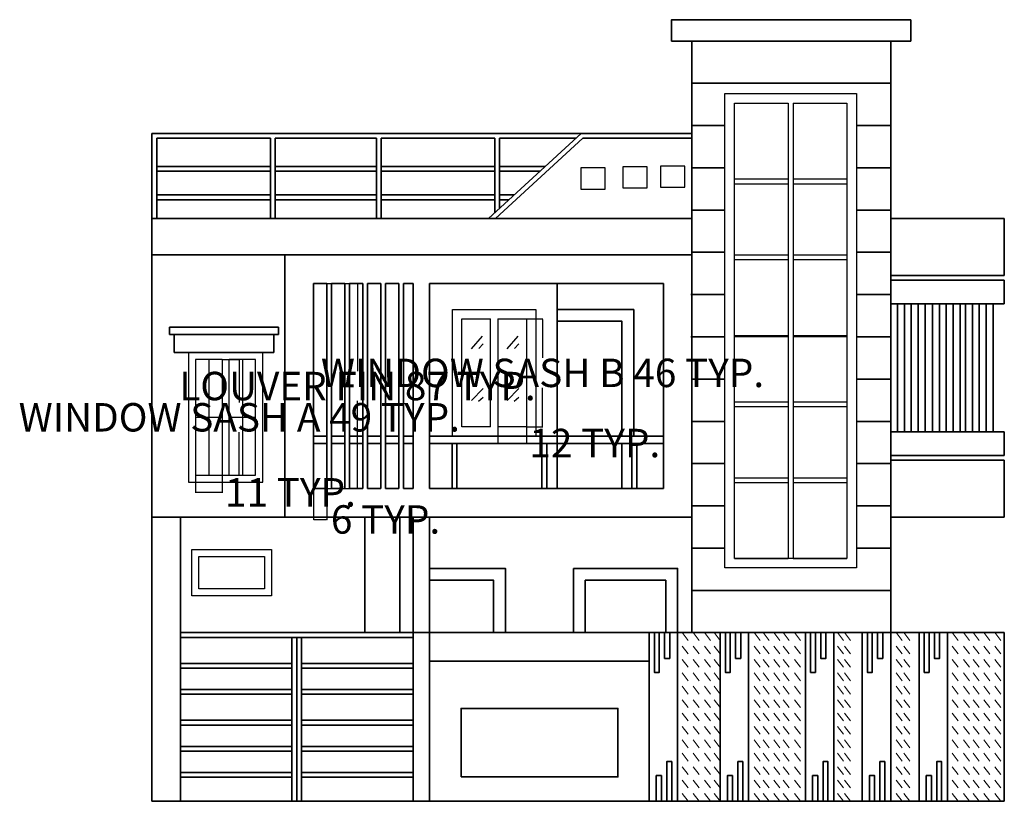
# Model space of a CAD drawing. Units: inches. Extents: x 2440 to 2856, y 337 to 667.
import ezdxf

# ---------------------------------------------------------------- set-up
doc = ezdxf.new("R2010")
doc.units = ezdxf.units.IN
doc.header["$MEASUREMENT"] = 0
for name, color, linetype, lineweight in [('A-ANNO-DIMS', 2, 'Continuous', 18), ('A-ELEV', 7, 'Continuous', 35), ('A-ELEV-PATT', 8, 'Continuous', 13), ('A-GLAZ', 4, 'Continuous', 25)]:
    doc.layers.add(name, color=color, linetype=linetype, lineweight=lineweight)
doc.styles.get("Standard").update_dxf_attribs({"font": 'arial.ttf'})
doc.dimstyles.get("Standard").update_dxf_attribs({"dimtxt": 12, "dimasz": 0.18, "dimexe": 0.18, "dimexo": 0.0625, "dimgap": 0.09, "dimtad": 0, "dimtih": 1, "dimtoh": 1, "dimdec": 0, "dimzin": 0, "dimdsep": 46, "dimlunit": 3, "dimtxsty": 'Standard', "dimcen": 0.09, "dimadec": 0, "dimazin": 0, "dimtfac": 1, "dimtdec": 0, "dimtofl": 0, "dimtmove": 0, "dimatfit": 3, "dimfxl": 1, "dimtolj": 1, "dimtzin": 0, "dimarcsym": 0})

# ---------------------------------------------------------------- blocks, each defined once
blk = doc.blocks.new('LOUVER-FIN')
for p, q in [((0, 0), (0, 86.66)), ((0, 86.66), (5.62, 86.66)), ((5.62, 0), (5.62, 86.66)), ((5.62, 0), (0, 0))]:
    blk.add_line(p, q)
blk = doc.blocks.new('WIN-SASH-A')
blk.add_line((11.19, 48.73), (11.19, 0))
blk.add_lwpolyline([(11.19, 48.73), (0, 48.73), (0, 0), (11.19, 0)])
blk = doc.blocks.new('WIN-SASH-B')
blk.add_line((0, 45.55), (0, 0))
blk.add_lwpolyline([(0, 45.55), (12.11, 45.55), (12.11, 0), (0, 0)])
blk = doc.blocks.new('*D4')
at = {"layer": 'A-ANNO-DIMS', "color": 0, "lineweight": -2, "transparency": 16777216}
for p, q in [((2569.72, 555.43), (2582.84, 555.43)), ((2582.66, 555.25), (2582.66, 518.4)), ((2582.66, 468.95), (2582.66, 505.8)), ((2569.72, 468.77), (2582.84, 468.77))]:
    blk.add_line(p, q, dxfattribs=at)
at = {"layer": 'A-ANNO-DIMS', "color": 0, "transparency": 16777216}
for points in [[(2582.63, 555.25), (2582.69, 555.25), (2582.66, 555.43)], [(2582.63, 468.95), (2582.69, 468.95), (2582.66, 468.77)]]:
    blk.add_solid(points, dxfattribs=at)
at = {"layer": 'Defpoints', "color": 0, "transparency": 16777216}
for p in [(2569.66, 555.43), (2582.66, 555.43), (2569.66, 468.77)]:
    blk.add_point(p, dxfattribs=at)
at = {"layer": 'A-ANNO-DIMS', "color": 0, "transparency": 16777216, "insert": (2582.66, 512.1), "char_height": 12, "attachment_point": 5}
blk.add_mtext('\\A1;LOUVER FIN 87 TYP.', dxfattribs=at)
blk = doc.blocks.new('*D5')
at = {"layer": 'A-ANNO-DIMS', "color": 0, "lineweight": -2, "transparency": 16777216}
for p, q in [((2564.04, 468.71), (2564.04, 455.59)), ((2569.66, 468.71), (2569.66, 455.59)), ((2564.22, 455.77), (2569.48, 455.77)), ((2569.66, 455.77), (2569.84, 455.77))]:
    blk.add_line(p, q, dxfattribs=at)
at = {"layer": 'A-ANNO-DIMS', "color": 0, "transparency": 16777216}
for points in [[(2564.22, 455.8), (2564.22, 455.74), (2564.04, 455.77)], [(2569.48, 455.8), (2569.48, 455.74), (2569.66, 455.77)]]:
    blk.add_solid(points, dxfattribs=at)
at = {"layer": 'Defpoints', "color": 0, "transparency": 16777216}
for p in [(2564.04, 468.77), (2569.66, 468.77), (2569.66, 455.77)]:
    blk.add_point(p, dxfattribs=at)
at = {"layer": 'A-ANNO-DIMS', "color": 0, "transparency": 16777216, "insert": (2594.51, 455.77), "char_height": 12, "attachment_point": 5}
blk.add_mtext('\\A1;6 TYP.', dxfattribs=at)
blk = doc.blocks.new('*D6')
at = {"layer": 'A-ANNO-DIMS', "color": 0, "lineweight": -2, "transparency": 16777216}
for p, q in [((2525.51, 523.26), (2532.93, 523.26)), ((2532.75, 523.08), (2532.75, 505.19)), ((2532.75, 474.71), (2532.75, 492.6)), ((2525.51, 474.53), (2532.93, 474.53))]:
    blk.add_line(p, q, dxfattribs=at)
at = {"layer": 'A-ANNO-DIMS', "color": 0, "transparency": 16777216}
for points in [[(2532.72, 523.08), (2532.78, 523.08), (2532.75, 523.26)], [(2532.72, 474.71), (2532.78, 474.71), (2532.75, 474.53)]]:
    blk.add_solid(points, dxfattribs=at)
at = {"layer": 'Defpoints', "color": 0, "transparency": 16777216}
for p in [(2525.45, 523.26), (2532.75, 523.26), (2525.45, 474.53)]:
    blk.add_point(p, dxfattribs=at)
at = {"layer": 'A-ANNO-DIMS', "color": 0, "transparency": 16777216, "insert": (2532.75, 498.9), "char_height": 12, "attachment_point": 5}
blk.add_mtext('\\A1;WINDOW SASH A 49 TYP.', dxfattribs=at)
blk = doc.blocks.new('*D7')
at = {"layer": 'A-ANNO-DIMS', "color": 0, "lineweight": -2, "transparency": 16777216}
for p, q in [((2514.26, 474.47), (2514.26, 467.04)), ((2525.45, 474.47), (2525.45, 467.04)), ((2514.44, 467.22), (2525.27, 467.22)), ((2525.45, 467.22), (2525.63, 467.22))]:
    blk.add_line(p, q, dxfattribs=at)
at = {"layer": 'A-ANNO-DIMS', "color": 0, "transparency": 16777216}
for points in [[(2514.44, 467.25), (2514.44, 467.19), (2514.26, 467.22)], [(2525.27, 467.25), (2525.27, 467.19), (2525.45, 467.22)]]:
    blk.add_solid(points, dxfattribs=at)
at = {"layer": 'Defpoints', "color": 0, "transparency": 16777216}
for p in [(2514.26, 474.53), (2525.45, 474.53), (2525.45, 467.22)]:
    blk.add_point(p, dxfattribs=at)
at = {"layer": 'A-ANNO-DIMS', "color": 0, "transparency": 16777216, "insert": (2554.36, 467.22), "char_height": 12, "attachment_point": 5}
blk.add_mtext('\\A1;11 TYP.', dxfattribs=at)
blk = doc.blocks.new('*D8')
at = {"layer": 'A-ANNO-DIMS', "color": 0, "lineweight": -2, "transparency": 16777216}
for p, q in [((2654.06, 540.42), (2661.01, 540.42)), ((2660.83, 540.24), (2660.83, 523.95)), ((2660.83, 495.05), (2660.83, 511.35)), ((2654.06, 494.87), (2661.01, 494.87))]:
    blk.add_line(p, q, dxfattribs=at)
at = {"layer": 'A-ANNO-DIMS', "color": 0, "transparency": 16777216}
for points in [[(2660.8, 540.24), (2660.86, 540.24), (2660.83, 540.42)], [(2660.8, 495.05), (2660.86, 495.05), (2660.83, 494.87)]]:
    blk.add_solid(points, dxfattribs=at)
at = {"layer": 'Defpoints', "color": 0, "transparency": 16777216}
for p in [(2654, 540.42), (2660.83, 540.42), (2654, 494.87)]:
    blk.add_point(p, dxfattribs=at)
at = {"layer": 'A-ANNO-DIMS', "color": 0, "transparency": 16777216, "insert": (2660.83, 517.65), "char_height": 12, "attachment_point": 5}
blk.add_mtext('\\A1;WINDOW SASH B 46 TYP.', dxfattribs=at)
blk = doc.blocks.new('*D9')
at = {"layer": 'A-ANNO-DIMS', "color": 0, "lineweight": -2, "transparency": 16777216}
for p, q in [((2641.89, 494.81), (2641.89, 487.86)), ((2654, 494.81), (2654, 487.86)), ((2642.07, 488.04), (2653.82, 488.04)), ((2654, 488.04), (2654.18, 488.04))]:
    blk.add_line(p, q, dxfattribs=at)
at = {"layer": 'A-ANNO-DIMS', "color": 0, "transparency": 16777216}
for points in [[(2642.07, 488.07), (2642.07, 488.01), (2641.89, 488.04)], [(2653.82, 488.07), (2653.82, 488.01), (2654, 488.04)]]:
    blk.add_solid(points, dxfattribs=at)
at = {"layer": 'Defpoints', "color": 0, "transparency": 16777216}
for p in [(2641.89, 494.87), (2654, 494.87), (2654, 488.04)]:
    blk.add_point(p, dxfattribs=at)
at = {"layer": 'A-ANNO-DIMS', "color": 0, "transparency": 16777216, "insert": (2682.91, 488.04), "char_height": 12, "attachment_point": 5}
blk.add_mtext('\\A1;12 TYP.', dxfattribs=at)

msp = doc.modelspace()

# ---------------------------------------------------------------- linework, layer by layer
at = {"layer": 'A-ELEV'}
for p, q in [((2807.87, 666.77), (2723.87, 666.77)), ((2816.4, 666.77), (2816.4, 657.77)), ((2723.87, 657.77), (2723.87, 407.97)), ((2807.87, 657.77), (2723.87, 657.77)), ((2807.87, 657.77), (2807.87, 456.77)), ((2807.87, 639.93), (2723.87, 639.93)), ((2737.87, 622.08), (2723.87, 622.08)), ((2807.87, 622.08), (2793.4, 622.08)), ((2723.87, 618.77), (2495.87, 618.77)), ((2495.87, 582.77), (2495.87, 618.77)), ((2497.87, 582.77), (2497.87, 616.77)), ((2545.87, 616.77), (2497.87, 616.77)), ((2545.87, 582.77), (2545.87, 616.77)), ((2547.87, 582.77), (2547.87, 616.77)), ((2590.66, 616.77), (2547.87, 616.77)), ((2590.66, 582.77), (2590.66, 616.77)), ((2592.66, 582.77), (2592.66, 616.77)), ((2640.66, 616.77), (2592.66, 616.77)), ((2637.96, 582.77), (2677.09, 618.77)), ((2640.66, 585.26), (2640.66, 616.77)), ((2640.91, 582.77), (2677.87, 616.77)), ((2642.66, 587.1), (2642.66, 616.77)), ((2674.91, 616.77), (2642.66, 616.77)), ((2723.87, 616.77), (2677.87, 616.77)), ((2723.87, 616.77), (2695.99, 616.77)), ((2545.87, 604.77), (2497.87, 604.77)), ((2590.66, 604.77), (2547.87, 604.77)), ((2640.66, 604.77), (2592.66, 604.77)), ((2661.87, 604.77), (2642.66, 604.77)), ((2737.87, 604.24), (2723.87, 604.24)), ((2807.87, 604.24), (2793.4, 604.24)), ((2545.87, 602.77), (2497.87, 602.77)), ((2590.66, 602.77), (2547.87, 602.77)), ((2640.66, 602.77), (2592.66, 602.77)), ((2659.7, 602.77), (2642.66, 602.77)), ((2545.87, 592.77), (2497.87, 592.77)), ((2545.87, 590.77), (2497.87, 590.77)), ((2590.66, 592.77), (2547.87, 592.77)), ((2590.66, 590.77), (2547.87, 590.77)), ((2640.66, 592.77), (2592.66, 592.77)), ((2640.66, 590.77), (2592.66, 590.77)), ((2648.83, 592.77), (2642.66, 592.77)), ((2646.65, 590.77), (2642.66, 590.77)), ((2737.87, 586.4), (2723.87, 586.4)), ((2807.87, 586.4), (2793.4, 586.4)), ((2495.87, 582.77), (2495.87, 456.77)), ((2723.87, 582.77), (2495.87, 582.77)), ((2675.87, 582.77), (2723.87, 582.77)), ((2723.87, 582.77), (2723.87, 567.43)), ((2855.87, 582.77), (2807.87, 582.77)), ((2855.87, 582.77), (2855.87, 558.77)), ((2552.04, 567.43), (2495.87, 567.43)), ((2723.87, 567.43), (2675.87, 567.43)), ((2737.87, 568.55), (2723.87, 568.55)), ((2807.87, 568.55), (2793.4, 568.55)), ((2855.87, 558.77), (2807.87, 558.77)), ((2602.13, 468.77), (2602.13, 555.43)), ((2602.13, 555.43), (2606.13, 555.43)), ((2606.13, 468.77), (2606.13, 555.43)), ((2613.13, 468.77), (2613.13, 555.43)), ((2613.13, 555.43), (2711.87, 555.43)), ((2666.96, 490.87), (2666.96, 555.43)), ((2711.87, 555.43), (2711.87, 468.77)), ((2855.87, 556.77), (2807.87, 556.77)), ((2855.87, 556.77), (2855.87, 546.77)), ((2737.87, 550.71), (2723.41, 550.71)), ((2807.87, 550.71), (2793.4, 550.71)), ((2855.87, 546.77), (2807.87, 546.77)), ((2807.87, 546.77), (2807.87, 492.77)), ((2810.77, 546.77), (2810.77, 492.77)), ((2813.68, 546.77), (2813.68, 492.77)), ((2816.59, 546.77), (2816.59, 492.77)), ((2819.49, 546.77), (2819.49, 492.77)), ((2822.4, 546.77), (2822.4, 492.77)), ((2825.53, 546.77), (2825.53, 492.77)), ((2828.44, 546.77), (2828.44, 492.77)), ((2831.35, 546.77), (2831.35, 492.77)), ((2834.25, 546.77), (2834.25, 492.77)), ((2837.16, 546.77), (2837.16, 492.77)), ((2839.49, 546.77), (2839.49, 492.77)), ((2842.4, 546.77), (2842.4, 492.77)), ((2845.3, 546.77), (2845.3, 492.77)), ((2848.21, 546.77), (2848.21, 492.77)), ((2851.11, 546.77), (2851.11, 492.77)), ((2666.96, 544.44), (2699.37, 544.44)), ((2699.37, 544.44), (2699.37, 490.87)), ((2549.28, 536.89), (2503.28, 536.89)), ((2503.28, 536.89), (2503.28, 533.89)), ((2549.28, 533.89), (2549.28, 536.89)), ((2549.28, 533.89), (2503.28, 533.89)), ((2505.28, 533.89), (2505.28, 526.26)), ((2547.28, 526.26), (2547.28, 533.89)), ((2737.87, 532.87), (2723.41, 532.87)), ((2807.87, 532.87), (2793.4, 532.87)), ((2505.28, 526.26), (2547.28, 526.26)), ((2737.87, 515.03), (2723.87, 515.03)), ((2807.87, 515.03), (2793.4, 515.03)), ((2737.87, 497.18), (2723.87, 497.18)), ((2807.87, 497.18), (2793.4, 497.18)), ((2569.66, 490.87), (2564.04, 490.87)), ((2577.28, 490.87), (2571.66, 490.87)), ((2584.9, 490.87), (2579.28, 490.87)), ((2592.51, 490.87), (2586.9, 490.87)), ((2600.13, 490.87), (2594.51, 490.87)), ((2606.13, 490.87), (2602.13, 490.87)), ((2711.87, 490.87), (2613.13, 490.87)), ((2855.87, 492.77), (2807.87, 492.77)), ((2855.87, 492.77), (2855.87, 482.77)), ((2569.66, 487.87), (2564.04, 487.87)), ((2577.28, 487.87), (2571.66, 487.87)), ((2584.9, 487.87), (2579.28, 487.87)), ((2592.51, 487.87), (2586.9, 487.87)), ((2600.13, 487.87), (2594.51, 487.87)), ((2606.13, 487.87), (2602.13, 487.87)), ((2711.87, 487.87), (2613.13, 487.87)), ((2622.59, 487.87), (2622.59, 468.77)), ((2624.59, 487.87), (2624.59, 468.77)), ((2660.59, 487.87), (2660.59, 468.77)), ((2662.59, 487.87), (2662.59, 468.77)), ((2698.59, 487.87), (2698.59, 468.77)), ((2700.59, 487.87), (2700.59, 468.77)), ((2855.87, 482.77), (2807.87, 482.77)), ((2737.87, 479.34), (2723.87, 479.34)), ((2807.87, 479.34), (2793.4, 479.34)), ((2855.87, 480.77), (2807.87, 480.77)), ((2855.87, 480.77), (2855.87, 456.77)), ((2606.13, 468.77), (2602.13, 468.77)), ((2711.87, 468.77), (2613.13, 468.77)), ((2737.87, 461.5), (2723.87, 461.5)), ((2807.87, 461.5), (2793.4, 461.5)), ((2495.87, 456.77), (2495.87, 336.77)), ((2723.87, 456.77), (2495.87, 456.77)), ((2507.87, 456.77), (2507.87, 336.77)), ((2606.13, 336.77), (2606.13, 456.77)), ((2613.13, 336.77), (2613.13, 456.77)), ((2807.87, 407.97), (2807.87, 456.77)), ((2855.87, 456.77), (2807.87, 456.77)), ((2737.87, 443.65), (2723.87, 443.65)), ((2807.87, 443.65), (2793.4, 443.65)), ((2807.87, 425.81), (2723.87, 425.81)), ((2606.13, 407.97), (2507.87, 407.97)), ((2855.87, 407.97), (2613.13, 407.97)), ((2705.87, 407.97), (2705.87, 336.77)), ((2717.87, 407.97), (2717.87, 336.77)), ((2807.87, 407.97), (2723.87, 407.97)), ((2735.87, 407.97), (2735.87, 336.77)), ((2747.87, 407.97), (2747.87, 336.77)), ((2771.87, 407.97), (2771.87, 336.77)), ((2783.87, 407.97), (2783.87, 336.77)), ((2795.87, 407.97), (2795.87, 336.77)), ((2807.87, 407.97), (2807.87, 336.77)), ((2819.87, 407.97), (2819.87, 336.77)), ((2831.87, 407.97), (2831.87, 336.77)), ((2855.87, 407.97), (2855.87, 336.77)), ((2606.13, 405.97), (2507.87, 405.97)), ((2555, 405.97), (2555, 336.77)), ((2557, 405.97), (2557, 336.77)), ((2559, 405.97), (2559, 336.77)), ((2705.87, 395.97), (2613.13, 395.97)), ((2555, 394.97), (2507.87, 394.97)), ((2555, 392.97), (2507.87, 392.97)), ((2606.13, 394.97), (2559, 394.97)), ((2606.13, 392.97), (2559, 392.97)), ((2555, 383.97), (2507.87, 383.97)), ((2606.13, 383.97), (2559, 383.97)), ((2555, 381.97), (2507.87, 381.97)), ((2606.13, 381.97), (2559, 381.97)), ((2555, 370.97), (2507.87, 370.97)), ((2606.13, 370.97), (2559, 370.97)), ((2555, 368.97), (2507.87, 368.97)), ((2606.13, 368.97), (2559, 368.97)), ((2555, 359.97), (2507.87, 359.97)), ((2555, 357.97), (2507.87, 357.97)), ((2606.13, 359.97), (2559, 359.97)), ((2606.13, 357.97), (2559, 357.97)), ((2555, 348.97), (2507.87, 348.97)), ((2555, 346.97), (2507.87, 346.97)), ((2606.13, 348.97), (2559, 348.97)), ((2606.13, 346.97), (2559, 346.97)), ((2495.87, 336.77), (2855.87, 336.77))]:
    msp.add_line(p, q, dxfattribs=at)
for points in [[(2723.87, 657.77), (2715.34, 657.77), (2715.34, 666.77), (2723.87, 666.77)], [(2807.87, 666.77), (2816.4, 666.77)], [(2816.4, 657.77), (2807.87, 657.77)], [(2694.37, 487.87), (2694.37, 468.77), (2666.96, 468.77), (2666.96, 539.44), (2694.37, 539.44), (2694.37, 490.87)], [(2585.72, 407.97), (2585.72, 456.77), (2600.54, 456.77), (2600.54, 407.97)], [(2613.13, 435.12), (2645.13, 435.12), (2645.13, 407.97), (2601.12, 407.97)], [(2606.12, 407.97), (2606.12, 430.12), (2606.13, 430.12)], [(2613.13, 430.12), (2640.13, 430.12), (2640.13, 407.97)], [(2678.86, 407.97), (2678.86, 430.12), (2712.87, 430.12), (2712.87, 407.97)], [(2600.54, 336.77), (2585.72, 336.77)]]:
    msp.add_lwpolyline(points, dxfattribs=at)
for points in [[(2723.87, 456.77), (2552.04, 456.77), (2552.04, 567.43), (2723.87, 567.43)], [(2673.86, 435.12), (2717.87, 435.12), (2717.87, 407.97), (2673.86, 407.97)], [(2708.06, 407.97), (2710.1, 407.97), (2710.1, 391.21), (2708.06, 391.21)], [(2712.37, 407.97), (2714.53, 407.97), (2714.53, 397.12), (2712.37, 397.12)], [(2738.06, 407.97), (2740.1, 407.97), (2740.1, 391.21), (2738.06, 391.21)], [(2742.37, 407.97), (2744.53, 407.97), (2744.53, 397.12), (2742.37, 397.12)], [(2774.06, 407.97), (2776.1, 407.97), (2776.1, 391.21), (2774.06, 391.21)], [(2778.37, 407.97), (2780.53, 407.97), (2780.53, 397.12), (2778.37, 397.12)], [(2798.06, 407.97), (2800.1, 407.97), (2800.1, 391.21), (2798.06, 391.21)], [(2802.37, 407.97), (2804.53, 407.97), (2804.53, 397.12), (2802.37, 397.12)], [(2822.06, 407.97), (2824.1, 407.97), (2824.1, 391.21), (2822.06, 391.21)], [(2826.37, 407.97), (2828.53, 407.97), (2828.53, 397.12), (2826.37, 397.12)], [(2626.43, 347.06), (2692.69, 347.06), (2692.69, 375.98), (2626.43, 375.98)], [(2715.37, 336.77), (2713.32, 336.77), (2713.32, 353.52), (2715.37, 353.52)], [(2745.37, 336.77), (2743.32, 336.77), (2743.32, 353.52), (2745.37, 353.52)], [(2781.37, 336.77), (2779.32, 336.77), (2779.32, 353.52), (2781.37, 353.52)], [(2805.37, 336.77), (2803.32, 336.77), (2803.32, 353.52), (2805.37, 353.52)], [(2829.37, 336.77), (2827.32, 336.77), (2827.32, 353.52), (2829.37, 353.52)], [(2711.05, 336.77), (2708.89, 336.77), (2708.89, 347.62), (2711.05, 347.62)], [(2741.05, 336.77), (2738.89, 336.77), (2738.89, 347.62), (2741.05, 347.62)], [(2777.05, 336.77), (2774.89, 336.77), (2774.89, 347.62), (2777.05, 347.62)], [(2801.05, 336.77), (2798.89, 336.77), (2798.89, 347.62), (2801.05, 347.62)], [(2825.05, 336.77), (2822.89, 336.77), (2822.89, 347.62), (2825.05, 347.62)]]:
    msp.add_lwpolyline(points, close=True, dxfattribs=at)
at = {"layer": 'A-ELEV-PATT'}
for p, q in [((2719.77, 407.97), (2722.3, 404.67)), ((2724.48, 407.97), (2727.02, 404.67)), ((2729.2, 407.97), (2731.73, 404.67)), ((2733.33, 407.97), (2735.87, 404.67)), ((2750.23, 407.97), (2752.76, 404.67)), ((2754.02, 407.97), (2756.56, 404.67)), ((2758.51, 407.97), (2761.04, 404.67)), ((2762.41, 407.97), (2764.95, 404.67)), ((2767.24, 407.97), (2769.77, 404.67)), ((2785.43, 407.97), (2787.96, 404.67)), ((2788.42, 407.97), (2790.95, 404.67)), ((2810.26, 407.97), (2812.79, 404.67)), ((2813.47, 407.97), (2816.01, 404.67)), ((2833.85, 407.97), (2836.39, 404.67)), ((2838.68, 407.97), (2841.22, 404.67)), ((2842.7, 407.97), (2845.24, 404.67)), ((2847.19, 407.97), (2849.72, 404.67)), ((2851.9, 407.97), (2854.43, 404.67)), ((2719.77, 402.31), (2722.3, 399.02)), ((2724.48, 402.31), (2727.02, 399.02)), ((2729.2, 402.31), (2731.73, 399.02)), ((2733.33, 402.31), (2735.87, 399.02)), ((2750.23, 402.31), (2752.76, 399.02)), ((2754.02, 402.31), (2756.56, 399.02)), ((2758.51, 402.31), (2761.04, 399.02)), ((2762.41, 402.31), (2764.95, 399.02)), ((2767.24, 402.31), (2769.77, 399.02)), ((2785.43, 402.31), (2787.96, 399.02)), ((2788.42, 402.31), (2790.95, 399.02)), ((2810.26, 402.31), (2812.79, 399.02)), ((2813.47, 402.31), (2816.01, 399.02)), ((2833.85, 402.31), (2836.39, 399.02)), ((2838.68, 402.31), (2841.22, 399.02)), ((2842.7, 402.31), (2845.24, 399.02)), ((2847.19, 402.31), (2849.72, 399.02)), ((2851.9, 402.31), (2854.43, 399.02)), ((2719.77, 396.65), (2722.3, 393.36)), ((2724.48, 396.65), (2727.02, 393.36)), ((2729.2, 396.65), (2731.73, 393.36)), ((2733.33, 396.65), (2735.87, 393.36)), ((2750.23, 396.65), (2752.76, 393.36)), ((2754.02, 396.65), (2756.56, 393.36)), ((2758.51, 396.65), (2761.04, 393.36)), ((2762.41, 396.65), (2764.95, 393.36)), ((2767.24, 396.65), (2769.77, 393.36)), ((2785.43, 396.65), (2787.96, 393.36)), ((2788.42, 396.65), (2790.95, 393.36)), ((2810.26, 396.65), (2812.79, 393.36)), ((2813.47, 396.65), (2816.01, 393.36)), ((2833.85, 396.65), (2836.39, 393.36)), ((2838.68, 396.65), (2841.22, 393.36)), ((2842.7, 396.65), (2845.24, 393.36)), ((2847.19, 396.65), (2849.72, 393.36)), ((2851.9, 396.65), (2854.43, 393.36)), ((2719.77, 390.99), (2722.3, 387.7)), ((2724.48, 390.99), (2727.02, 387.7)), ((2729.2, 390.99), (2731.73, 387.7)), ((2733.33, 390.99), (2735.87, 387.7)), ((2750.23, 390.99), (2752.76, 387.7)), ((2754.02, 390.99), (2756.56, 387.7)), ((2758.51, 390.99), (2761.04, 387.7)), ((2762.41, 390.99), (2764.95, 387.7)), ((2767.24, 390.99), (2769.77, 387.7)), ((2785.43, 390.99), (2787.96, 387.7)), ((2788.42, 390.99), (2790.95, 387.7)), ((2810.26, 390.99), (2812.79, 387.7)), ((2813.47, 390.99), (2816.01, 387.7)), ((2833.85, 390.99), (2836.39, 387.7)), ((2838.68, 390.99), (2841.22, 387.7)), ((2842.7, 390.99), (2845.24, 387.7)), ((2847.19, 390.99), (2849.72, 387.7)), ((2851.9, 390.99), (2854.43, 387.7)), ((2719.77, 385.33), (2722.3, 382.04)), ((2724.48, 385.33), (2727.02, 382.04)), ((2729.2, 385.33), (2731.73, 382.04)), ((2733.33, 385.33), (2735.87, 382.04)), ((2750.23, 385.33), (2752.76, 382.04)), ((2754.02, 385.33), (2756.56, 382.04)), ((2758.51, 385.33), (2761.04, 382.04)), ((2762.41, 385.33), (2764.95, 382.04)), ((2767.24, 385.33), (2769.77, 382.04)), ((2785.43, 385.33), (2787.96, 382.04)), ((2788.42, 385.33), (2790.95, 382.04)), ((2810.26, 385.33), (2812.79, 382.04)), ((2813.47, 385.33), (2816.01, 382.04)), ((2833.85, 385.33), (2836.39, 382.04)), ((2838.68, 385.33), (2841.22, 382.04)), ((2842.7, 385.33), (2845.24, 382.04)), ((2847.19, 385.33), (2849.72, 382.04)), ((2851.9, 385.33), (2854.43, 382.04)), ((2719.77, 379.67), (2722.3, 376.38)), ((2724.48, 379.67), (2727.02, 376.38)), ((2729.2, 379.67), (2731.73, 376.38)), ((2733.33, 379.67), (2735.87, 376.38)), ((2750.23, 379.67), (2752.76, 376.38)), ((2754.02, 379.67), (2756.56, 376.38)), ((2758.51, 379.67), (2761.04, 376.38)), ((2762.41, 379.67), (2764.95, 376.38)), ((2767.24, 379.67), (2769.77, 376.38)), ((2785.43, 379.67), (2787.96, 376.38)), ((2788.42, 379.67), (2790.95, 376.38)), ((2810.26, 379.67), (2812.79, 376.38)), ((2813.47, 379.67), (2816.01, 376.38)), ((2833.85, 379.67), (2836.39, 376.38)), ((2838.68, 379.67), (2841.22, 376.38)), ((2842.7, 379.67), (2845.24, 376.38)), ((2847.19, 379.67), (2849.72, 376.38)), ((2851.9, 379.67), (2854.43, 376.38)), ((2719.77, 374.01), (2722.3, 370.72)), ((2724.48, 374.01), (2727.02, 370.72)), ((2729.2, 374.01), (2731.73, 370.72)), ((2733.33, 374.01), (2735.87, 370.72)), ((2750.23, 374.01), (2752.76, 370.72)), ((2754.02, 374.01), (2756.56, 370.72)), ((2758.51, 374.01), (2761.04, 370.72)), ((2762.41, 374.01), (2764.95, 370.72)), ((2767.24, 374.01), (2769.77, 370.72)), ((2785.43, 374.01), (2787.96, 370.72)), ((2788.42, 374.01), (2790.95, 370.72)), ((2810.26, 374.01), (2812.79, 370.72)), ((2813.47, 374.01), (2816.01, 370.72)), ((2833.85, 374.01), (2836.39, 370.72)), ((2838.68, 374.01), (2841.22, 370.72)), ((2842.7, 374.01), (2845.24, 370.72)), ((2847.19, 374.01), (2849.72, 370.72)), ((2851.9, 374.01), (2854.43, 370.72)), ((2719.77, 368.36), (2722.3, 365.06)), ((2724.48, 368.36), (2727.02, 365.06)), ((2729.2, 368.36), (2731.73, 365.06)), ((2733.33, 368.36), (2735.87, 365.06)), ((2750.23, 368.36), (2752.76, 365.06)), ((2754.02, 368.36), (2756.56, 365.06)), ((2758.51, 368.36), (2761.04, 365.06)), ((2762.41, 368.36), (2764.95, 365.06)), ((2767.24, 368.36), (2769.77, 365.06)), ((2785.43, 368.36), (2787.96, 365.06)), ((2788.42, 368.36), (2790.95, 365.06)), ((2810.26, 368.36), (2812.79, 365.06)), ((2813.47, 368.36), (2816.01, 365.06)), ((2833.85, 368.36), (2836.39, 365.06)), ((2838.68, 368.36), (2841.22, 365.06)), ((2842.7, 368.36), (2845.24, 365.06)), ((2847.19, 368.36), (2849.72, 365.06)), ((2851.9, 368.36), (2854.43, 365.06)), ((2719.77, 362.7), (2722.3, 359.4)), ((2724.48, 362.7), (2727.02, 359.4)), ((2729.2, 362.7), (2731.73, 359.4)), ((2733.33, 362.7), (2735.87, 359.4)), ((2750.23, 362.7), (2752.76, 359.4)), ((2754.02, 362.7), (2756.56, 359.4)), ((2758.51, 362.7), (2761.04, 359.4)), ((2762.41, 362.7), (2764.95, 359.4)), ((2767.24, 362.7), (2769.77, 359.4)), ((2785.43, 362.7), (2787.96, 359.4)), ((2788.42, 362.7), (2790.95, 359.4)), ((2810.26, 362.7), (2812.79, 359.4)), ((2813.47, 362.7), (2816.01, 359.4)), ((2833.85, 362.7), (2836.39, 359.4)), ((2838.68, 362.7), (2841.22, 359.4)), ((2842.7, 362.7), (2845.24, 359.4)), ((2847.19, 362.7), (2849.72, 359.4)), ((2851.9, 362.7), (2854.43, 359.4)), ((2719.77, 357.04), (2722.3, 353.75)), ((2724.48, 357.04), (2727.02, 353.75)), ((2729.2, 357.04), (2731.73, 353.75)), ((2733.33, 357.04), (2735.87, 353.75)), ((2750.23, 357.04), (2752.76, 353.75)), ((2754.02, 357.04), (2756.56, 353.75)), ((2758.51, 357.04), (2761.04, 353.75)), ((2762.41, 357.04), (2764.95, 353.75)), ((2767.24, 357.04), (2769.77, 353.75)), ((2785.43, 357.04), (2787.96, 353.75)), ((2788.42, 357.04), (2790.95, 353.75)), ((2810.26, 357.04), (2812.79, 353.75)), ((2813.47, 357.04), (2816.01, 353.75)), ((2833.85, 357.04), (2836.39, 353.75)), ((2838.68, 357.04), (2841.22, 353.75)), ((2842.7, 357.04), (2845.24, 353.75)), ((2847.19, 357.04), (2849.72, 353.75)), ((2851.9, 357.04), (2854.43, 353.75)), ((2719.77, 351.38), (2722.3, 348.09)), ((2724.48, 351.38), (2727.02, 348.09)), ((2729.2, 351.38), (2731.73, 348.09)), ((2733.33, 351.38), (2735.87, 348.09)), ((2750.23, 351.38), (2752.76, 348.09)), ((2754.02, 351.38), (2756.56, 348.09)), ((2758.51, 351.38), (2761.04, 348.09)), ((2762.41, 351.38), (2764.95, 348.09)), ((2767.24, 351.38), (2769.77, 348.09)), ((2785.43, 351.38), (2787.96, 348.09)), ((2788.42, 351.38), (2790.95, 348.09)), ((2810.26, 351.38), (2812.79, 348.09)), ((2813.47, 351.38), (2816.01, 348.09)), ((2833.85, 351.38), (2836.39, 348.09)), ((2838.68, 351.38), (2841.22, 348.09)), ((2842.7, 351.38), (2845.24, 348.09)), ((2847.19, 351.38), (2849.72, 348.09)), ((2851.9, 351.38), (2854.43, 348.09)), ((2719.77, 345.72), (2722.3, 342.43)), ((2724.48, 345.72), (2727.02, 342.43)), ((2729.2, 345.72), (2731.73, 342.43)), ((2733.33, 345.72), (2735.87, 342.43)), ((2750.23, 345.72), (2752.76, 342.43)), ((2754.02, 345.72), (2756.56, 342.43)), ((2758.51, 345.72), (2761.04, 342.43)), ((2762.41, 345.72), (2764.95, 342.43)), ((2767.24, 345.72), (2769.77, 342.43)), ((2785.43, 345.72), (2787.96, 342.43)), ((2788.42, 345.72), (2790.95, 342.43)), ((2810.26, 345.72), (2812.79, 342.43)), ((2813.47, 345.72), (2816.01, 342.43)), ((2833.85, 345.72), (2836.39, 342.43)), ((2838.68, 345.72), (2841.22, 342.43)), ((2842.7, 345.72), (2845.24, 342.43)), ((2847.19, 345.72), (2849.72, 342.43)), ((2851.9, 345.72), (2854.43, 342.43)), ((2719.77, 340.06), (2722.3, 336.77)), ((2724.48, 340.06), (2727.02, 336.77)), ((2729.2, 340.06), (2731.73, 336.77)), ((2733.33, 340.06), (2735.87, 336.77)), ((2750.23, 340.06), (2752.76, 336.77)), ((2754.02, 340.06), (2756.56, 336.77)), ((2758.51, 340.06), (2761.04, 336.77)), ((2762.41, 340.06), (2764.95, 336.77)), ((2767.24, 340.06), (2769.77, 336.77)), ((2785.43, 340.06), (2787.96, 336.77)), ((2788.42, 340.06), (2790.95, 336.77)), ((2810.26, 340.06), (2812.79, 336.77)), ((2813.47, 340.06), (2816.01, 336.77)), ((2833.85, 340.06), (2836.39, 336.77)), ((2838.68, 340.06), (2841.22, 336.77)), ((2842.7, 340.06), (2845.24, 336.77)), ((2847.19, 340.06), (2849.72, 336.77)), ((2851.9, 340.06), (2854.43, 336.77))]:
    msp.add_line(p, q, dxfattribs=at)
at = {"layer": 'A-GLAZ'}
for p, q in [((2741.87, 631.57), (2764.64, 631.57)), ((2741.87, 439.35), (2741.87, 631.57)), ((2764.64, 631.57), (2764.64, 439.35)), ((2766.64, 631.57), (2766.64, 439.35)), ((2766.64, 631.57), (2789.4, 631.57)), ((2789.4, 631.57), (2789.4, 439.35)), ((2741.87, 599.54), (2764.64, 599.54)), ((2766.64, 599.54), (2789.4, 599.54)), ((2741.87, 597.54), (2764.64, 597.54)), ((2766.64, 597.54), (2789.4, 597.54)), ((2741.87, 567.5), (2764.64, 567.5)), ((2766.64, 567.5), (2789.4, 567.5)), ((2741.87, 565.5), (2764.64, 565.5)), ((2766.64, 565.5), (2789.4, 565.5)), ((2630.84, 527.78), (2635.45, 533.21)), ((2645.95, 527.78), (2650.56, 533.21)), ((2741.87, 533.46), (2764.64, 533.46)), ((2764.64, 532.87), (2741.87, 532.87)), ((2766.64, 533.46), (2789.4, 533.46)), ((2789.4, 532.87), (2766.64, 532.87)), ((2633.91, 527.89), (2635.68, 529.9)), ((2649.02, 527.89), (2650.79, 529.9)), ((2519.85, 523.26), (2519.85, 474.53)), ((2534.04, 523.26), (2534.04, 474.53)), ((2630.84, 506.05), (2635.68, 511.01)), ((2645.95, 506.05), (2650.79, 511.01)), ((2633.79, 505.7), (2635.68, 507.35)), ((2648.9, 505.7), (2650.79, 507.35)), ((2741.87, 505.43), (2764.64, 505.43)), ((2741.87, 503.43), (2764.64, 503.43)), ((2766.64, 505.43), (2789.4, 505.43)), ((2766.64, 503.43), (2789.4, 503.43)), ((2514.26, 498.9), (2525.45, 498.9)), ((2528.45, 498.9), (2539.63, 498.9)), ((2741.87, 473.39), (2764.64, 473.39)), ((2741.87, 471.39), (2764.64, 471.39)), ((2766.64, 473.39), (2789.4, 473.39)), ((2766.64, 471.39), (2789.4, 471.39)), ((2789.4, 439.35), (2741.87, 439.35)), ((2741.87, 439.35), (2764.64, 439.35)), ((2766.64, 439.35), (2789.4, 439.35))]:
    msp.add_line(p, q, dxfattribs=at)
for points in [[(2737.87, 635.57), (2793.4, 635.57), (2793.4, 435.35), (2737.87, 435.35)], [(2687.26, 604.19), (2677, 604.19), (2677, 595.26), (2687.26, 595.26)], [(2705, 604.67), (2694.74, 604.67), (2694.74, 595.74), (2705, 595.74)], [(2720.96, 604.98), (2710.71, 604.98), (2710.71, 596.05), (2720.96, 596.05)], [(2622.78, 544.42), (2658, 544.42), (2658, 490.87), (2622.78, 490.87)], [(2511.26, 471.53), (2542.63, 471.53), (2542.63, 526.26), (2511.26, 526.26)], [(2512.67, 443.1), (2546.36, 443.1), (2546.36, 423.46), (2512.67, 423.46)], [(2515.67, 440.1), (2543.36, 440.1), (2543.36, 426.46), (2515.67, 426.46)]]:
    msp.add_lwpolyline(points, close=True, dxfattribs=at)

# ---------------------------------------------------------------- block references
at = {"layer": 'A-ELEV'}
msp.add_blockref('LOUVER-FIN', (2564.05, 468.77), dxfattribs=at)
at = {"layer": 'A-ELEV', "rotation": 180}
for p in [(2577.28, 555.43), (2584.9, 555.43), (2592.51, 555.43), (2600.13, 555.43)]:
    msp.add_blockref('LOUVER-FIN', p, dxfattribs=at)
at = {"layer": 'A-GLAZ', "rotation": 180}
for name, p in [('WIN-SASH-B', (2638.89, 540.42)), ('WIN-SASH-A', (2539.63, 523.26))]:
    msp.add_blockref(name, p, dxfattribs=at)
at = {"layer": 'A-GLAZ'}
for name, p in [('WIN-SASH-B', (2641.89, 494.87)), ('WIN-SASH-A', (2514.26, 474.53))]:
    msp.add_blockref(name, p, dxfattribs=at)

# ---------------------------------------------------------------- dimensions: what is measured, and where the dimension line sits
at = {"layer": 'A-ANNO-DIMS'}
for base, p1, p2, text, picture, middle in [((2660.83, 540.42), (2654, 494.87), (2654, 540.42), 'WINDOW SASH B <> TYP.', '*D8', (2660.83, 517.65)), ((2582.66, 555.43), (2569.66, 468.77), (2569.66, 555.43), 'LOUVER FIN <> TYP.', '*D4', (2582.66, 512.1)), ((2532.75, 523.26), (2525.45, 474.53), (2525.45, 523.26), 'WINDOW SASH A <> TYP.', '*D6', (2532.75, 498.9))]:
    dim = msp.add_linear_dim(base=base, p1=p1, p2=p2, angle=90, text=text, dimstyle='Standard', override={"dimdec": 0, "dimlfac": 1, "dimrnd": 0, "dimzin": 0, "dimdsep": 46, "dimlunit": 2}, dxfattribs=at)
    dim.commit()
    dim.dimension.update_dxf_attribs({"geometry": picture, "text_midpoint": middle})
for base, p1, p2, picture, middle in [((2654, 488.04), (2641.89, 494.87), (2654, 494.87), '*D9', (2682.91, 488.04)), ((2525.45, 467.22), (2514.26, 474.53), (2525.45, 474.53), '*D7', (2554.36, 467.22)), ((2569.66, 455.77), (2564.04, 468.77), (2569.66, 468.77), '*D5', (2594.51, 455.77))]:
    dim = msp.add_linear_dim(base=base, p1=p1, p2=p2, text='<> TYP.', dimstyle='Standard', override={"dimdec": 0, "dimlfac": 1, "dimrnd": 0, "dimzin": 0, "dimdsep": 46, "dimlunit": 2}, dxfattribs=at)
    dim.commit()
    dim.dimension.update_dxf_attribs({"geometry": picture, "text_midpoint": middle})

doc.saveas('drawing.dxf')
